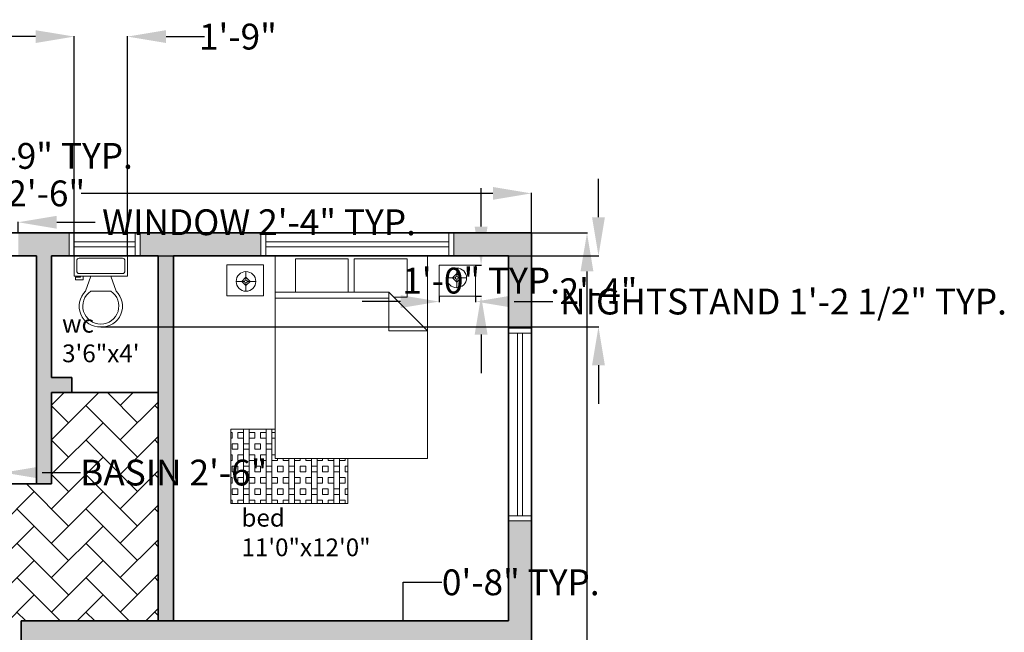
# Model space of a CAD drawing. Units: inches. Extents: x 1031 to 1706, y 87 to 654.
# Tile 4 of 4: x 1318 to 1706, y 413 to 654. Entities that reach past the tile are written whole.
import ezdxf

# ---------------------------------------------------------------- set-up
doc = ezdxf.new("R2010")
doc.units = ezdxf.units.IN
doc.header["$MEASUREMENT"] = 0
for name, color, linetype, lineweight in [('A-ANNO-DIMS', 2, 'Continuous', 18), ('A-AREA-IDEN', 7, 'Continuous', 25), ('A-FLOR-FIXT', 114, 'Continuous', 18), ('A-FLOR-PATT', 152, 'Continuous', 13), ('A-FURN', 215, 'Continuous', 18), ('A-GLAZ', 4, 'Continuous', 18), ('A-WALL', 7, 'Continuous', 35), ('A-WALL-PATT', 18, 'Continuous', 13)]:
    doc.layers.add(name, color=color, linetype=linetype, lineweight=lineweight)
doc.styles.get("Standard").update_dxf_attribs({"font": 'arial.ttf'})
doc.dimstyles.get("Standard").update_dxf_attribs({"dimtxt": 10.18, "dimasz": 15.18, "dimexe": 0.18, "dimexo": 0.0625, "dimgap": 0.09, "dimtad": 0, "dimtih": 1, "dimtoh": 1, "dimdec": 0, "dimzin": 0, "dimdsep": 46, "dimlunit": 3, "dimtxsty": 'Standard', "dimcen": 0.09, "dimadec": 0, "dimazin": 0, "dimtfac": 1, "dimtdec": 0, "dimtofl": 0, "dimtmove": 0, "dimatfit": 3, "dimfxl": 1, "dimtolj": 1, "dimtzin": 0, "dimarcsym": 0})

# ---------------------------------------------------------------- blocks, each defined once
blk = doc.blocks.new('Bed - Queen')
for p, q in [((0, -80.00003), (0, 0)), ((0, 0), (59.99999, 0)), ((59.99999, 0), (59.99999, -80.00003)), ((7.99999, -1.2), (28.79998, -1.2)), ((7.99999, -14.4), (7.99999, -1.2)), ((28.79998, -1.2), (28.79998, -14.4)), ((31.19999, -1.2), (51.99999, -1.2)), ((31.19999, -14.4), (31.19999, -1.2)), ((51.99999, -1.2), (51.99999, -16.4)), ((0, -14.4), (44.8, -14.4)), ((59.99999, -29.6), (44.8, -14.4)), ((44.8, -14.4), (44.8, -29.6)), ((44.8, -16.8), (0, -16.8)), ((51.99999, -16.4), (46.79936, -16.4)), ((44.8, -29.6), (59.99999, -29.6)), ((59.99999, -80.00003), (0, -80.00003))]:
    blk.add_line(p, q)
blk = doc.blocks.new('Lamp - Table')
for p, q in [((-1, 0), (-7, 0)), ((0, 3), (-3, 0)), ((-3, 0), (0, -3)), ((0, 7), (0, 1)), ((3, 0), (0, 3)), ((0, -3), (3, 0)), ((1, 0), (7, 0)), ((0, -1), (0, -7))]:
    blk.add_line(p, q)
for radius in [7, 1]:
    blk.add_circle((0, 0), radius)
blk = doc.blocks.new('*U11')
for p, q in [((9.5, -6), (9.5, -2)), ((-10, -8.5), (-8, -8.5)), ((-10, -9.5), (-10, -8.5)), ((-7, -9.5), (-10, -9.5)), ((-8, -8.5), (-8, -8)), ((-7, -8), (-7, -9.5)), ((-4, -8), (-6, -14)), ((4, -8), (6, -14)), ((4, -14), (-4, -14))]:
    blk.add_line(p, q)
blk.add_lwpolyline([(10.5, -8), (10.5, 0), (-10.5, 0), (-10.5, -8)], close=True)
for points in [[(-9.5, -2), (-9.5, -6)], [(8.5, -1), (-8.5, -1)], [(-8.5, -7), (8.5, -7)]]:
    blk.add_lwpolyline(points)
for centre, radius, start, end in [((-8.625, -1.875), 0.8839, 81.8699, 188.1301), ((8.625, -1.875), 0.8839, 351.8699, 98.1301), ((-8.625, -6.125), 0.8839, 171.869898, 278.1301), ((8.625, -6.125), 0.8839, 261.8699, 8.1301), ((-0.4772, -19.9188), 8.0953, 133.01722, 273.38), ((0.0374, -19.8731), 7.127, 124.50543, 269.7), ((-0.0373, -19.8731), 7.127, 270.3, 55.4946), ((0.4773, -19.9188), 8.0953, 266.62, 46.9828)]:
    blk.add_arc(centre, radius, start, end)
blk = doc.blocks.new('*D12')
at = {"layer": 'A-ANNO-DIMS', "color": 0, "lineweight": -2, "transparency": 16777216}
for p, q in [((1129.6, 570.46), (1129.6, 586.16)), ((1144.78, 585.98), (1307.03, 585.98)), ((1504.42, 585.98), (1342.17, 585.98)), ((1519.6, 570.46), (1519.6, 586.16))]:
    blk.add_line(p, q, dxfattribs=at)
at = {"layer": 'A-ANNO-DIMS', "color": 0, "transparency": 16777216}
for points in [[(1144.78, 588.51), (1144.78, 583.45), (1129.6, 585.98)], [(1504.42, 588.51), (1504.42, 583.45), (1519.6, 585.98)]]:
    blk.add_solid(points, dxfattribs=at)
at = {"layer": 'Defpoints', "color": 0, "transparency": 16777216}
for p in [(1519.6, 585.98), (1129.6, 570.4), (1519.6, 570.4)]:
    blk.add_point(p, dxfattribs=at)
at = {"layer": 'A-ANNO-DIMS', "color": 0, "transparency": 16777216, "insert": (1324.6, 585.98), "char_height": 10.18, "attachment_point": 5}
blk.add_mtext('\\A1;32\'-6"', dxfattribs=at)
blk = doc.blocks.new('*D14')
at = {"layer": 'A-ANNO-DIMS', "color": 0, "lineweight": -2, "transparency": 16777216}
for p, q in [((1519.66, 570.4), (1541.66, 570.4)), ((1541.48, 555.22), (1541.48, 383.69)), ((1541.48, 201.58), (1541.48, 373.11)), ((1519.66, 186.4), (1541.66, 186.4))]:
    blk.add_line(p, q, dxfattribs=at)
at = {"layer": 'A-ANNO-DIMS', "color": 0, "transparency": 16777216}
for points in [[(1538.95, 555.22), (1544.01, 555.22), (1541.48, 570.4)], [(1538.95, 201.58), (1544.01, 201.58), (1541.48, 186.4)]]:
    blk.add_solid(points, dxfattribs=at)
at = {"layer": 'Defpoints', "color": 0, "transparency": 16777216}
for p in [(1519.6, 570.4), (1519.6, 186.4), (1541.48, 186.4)]:
    blk.add_point(p, dxfattribs=at)
at = {"layer": 'A-ANNO-DIMS', "color": 0, "transparency": 16777216, "insert": (1541.48, 378.4), "char_height": 10.18, "attachment_point": 5}
blk.add_mtext("\\A1;32'", dxfattribs=at)
blk = doc.blocks.new('WIN-72IN')
for p, q in [((0, 0), (0, 9)), ((2, 0), (2, 9)), ((74, 0), (74, 9)), ((76, 0), (76, 9)), ((2, 5.5), (74, 5.5)), ((2, 3.5), (74, 3.5))]:
    blk.add_line(p, q)
blk = doc.blocks.new('WIN-24IN')
for p, q in [((0, 0), (0, 9)), ((2, 0), (2, 9)), ((26, 0), (26, 9)), ((28, 0), (28, 9)), ((2, 5.5), (26, 5.5)), ((2, 3.5), (26, 3.5))]:
    blk.add_line(p, q)
blk = doc.blocks.new('NIGHTSTAND-RECT')
blk.add_lwpolyline([(0, 12.21), (14.36, 12.21), (14.36, 0), (0, 0)], close=True)
blk = doc.blocks.new('*D20')
at = {"layer": 'A-ANNO-DIMS', "color": 0, "lineweight": -2, "transparency": 16777216}
for p, q in [((1274.24, 574.6), (1259.06, 574.6)), ((1289.42, 570.46), (1289.42, 574.78)), ((1317.42, 570.46), (1317.42, 574.78)), ((1332.6, 574.6), (1347.78, 574.6))]:
    blk.add_line(p, q, dxfattribs=at)
at = {"layer": 'A-ANNO-DIMS', "color": 0, "transparency": 16777216}
for points in [[(1274.24, 577.13), (1274.24, 572.07), (1289.42, 574.6)], [(1332.6, 577.13), (1332.6, 572.07), (1317.42, 574.6)]]:
    blk.add_solid(points, dxfattribs=at)
at = {"layer": 'Defpoints', "color": 0, "transparency": 16777216}
for p in [(1317.42, 574.6), (1289.42, 570.4), (1317.42, 570.4)]:
    blk.add_point(p, dxfattribs=at)
at = {"layer": 'A-ANNO-DIMS', "color": 0, "transparency": 16777216, "insert": (1412.28, 574.6), "char_height": 10.18, "attachment_point": 5}
blk.add_mtext('\\A1;WINDOW 2\'-4" TYP.', dxfattribs=at)
blk = doc.blocks.new('*D21')
at = {"layer": 'A-ANNO-DIMS', "color": 0, "lineweight": -2, "transparency": 16777216}
for p, q in [((1285.22, 585.58), (1285.22, 600.76)), ((1285.22, 600.76), (1300.4, 600.76)), ((1289.36, 570.4), (1285.04, 570.4)), ((1289.36, 561.4), (1285.04, 561.4)), ((1285.22, 546.22), (1285.22, 531.04))]:
    blk.add_line(p, q, dxfattribs=at)
at = {"layer": 'A-ANNO-DIMS', "color": 0, "transparency": 16777216}
for points in [[(1282.69, 585.58), (1287.75, 585.58), (1285.22, 570.4)], [(1282.69, 546.22), (1287.75, 546.22), (1285.22, 561.4)]]:
    blk.add_solid(points, dxfattribs=at)
at = {"layer": 'Defpoints', "color": 0, "transparency": 16777216}
for p in [(1285.22, 570.4), (1289.42, 570.4), (1289.42, 561.4)]:
    blk.add_point(p, dxfattribs=at)
at = {"layer": 'A-ANNO-DIMS', "color": 0, "transparency": 16777216, "insert": (1331.51, 600.76), "char_height": 10.18, "attachment_point": 5}
blk.add_mtext('\\A1;0\'-9" TYP.', dxfattribs=at)
blk = doc.blocks.new('*D24')
at = {"layer": 'A-ANNO-DIMS', "color": 0, "lineweight": -2, "transparency": 16777216}
for p, q in [((1468.08, 543.32), (1452.9, 543.32)), ((1483.26, 545.42), (1483.26, 543.14)), ((1497.62, 545.42), (1497.62, 543.14)), ((1512.8, 543.32), (1527.98, 543.32))]:
    blk.add_line(p, q, dxfattribs=at)
at = {"layer": 'A-ANNO-DIMS', "color": 0, "transparency": 16777216}
for points in [[(1468.08, 545.85), (1468.08, 540.79), (1483.26, 543.32)], [(1512.8, 545.85), (1512.8, 540.79), (1497.62, 543.32)]]:
    blk.add_solid(points, dxfattribs=at)
at = {"layer": 'Defpoints', "color": 0, "transparency": 16777216}
for p in [(1483.26, 545.48), (1497.62, 545.48), (1497.62, 543.32)]:
    blk.add_point(p, dxfattribs=at)
at = {"layer": 'A-ANNO-DIMS', "color": 0, "transparency": 16777216, "insert": (1618.9, 543.32), "char_height": 10.18, "attachment_point": 5}
blk.add_mtext('\\A1;NIGHTSTAND 1\'-2 1/2" TYP.', dxfattribs=at)
blk = doc.blocks.new('*D25')
at = {"layer": 'A-ANNO-DIMS', "color": 0, "lineweight": -2, "transparency": 16777216}
for p, q in [((1499.77, 572.86), (1499.77, 588.04)), ((1497.68, 557.68), (1499.95, 557.68)), ((1497.68, 545.48), (1499.95, 545.48)), ((1499.77, 530.3), (1499.77, 515.12))]:
    blk.add_line(p, q, dxfattribs=at)
at = {"layer": 'A-ANNO-DIMS', "color": 0, "transparency": 16777216}
for points in [[(1497.24, 572.86), (1502.3, 572.86), (1499.77, 557.68)], [(1497.24, 530.3), (1502.3, 530.3), (1499.77, 545.48)]]:
    blk.add_solid(points, dxfattribs=at)
at = {"layer": 'Defpoints', "color": 0, "transparency": 16777216}
for p in [(1497.62, 557.68), (1499.77, 557.68), (1497.62, 545.48)]:
    blk.add_point(p, dxfattribs=at)
at = {"layer": 'A-ANNO-DIMS', "color": 0, "transparency": 16777216, "insert": (1499.77, 551.58), "char_height": 10.18, "attachment_point": 5}
blk.add_mtext('\\A1;1\'-0" TYP.', dxfattribs=at)
blk = doc.blocks.new('*D26')
at = {"layer": 'A-ANNO-DIMS', "color": 0, "lineweight": -2, "transparency": 16777216}
for p, q in [((1455.08, 403.42), (1439.9, 403.42)), ((1470.26, 402.32), (1470.26, 403.6)), ((1478.02, 402.32), (1478.02, 403.6)), ((1493.2, 403.42), (1508.38, 403.42))]:
    blk.add_line(p, q, dxfattribs=at)
at = {"layer": 'A-ANNO-DIMS', "color": 0, "transparency": 16777216}
for points in [[(1455.08, 405.95), (1455.08, 400.89), (1470.26, 403.42)], [(1493.2, 405.95), (1493.2, 400.89), (1478.02, 403.42)]]:
    blk.add_solid(points, dxfattribs=at)
at = {"layer": 'Defpoints', "color": 0, "transparency": 16777216}
for p in [(1478.02, 403.42), (1470.26, 402.26), (1478.02, 402.26)]:
    blk.add_point(p, dxfattribs=at)
at = {"layer": 'A-ANNO-DIMS', "color": 0, "transparency": 16777216, "insert": (1560.61, 403.42), "char_height": 10.18, "attachment_point": 5}
blk.add_mtext('\\A1;LAMP 0\'-8" TYP.', dxfattribs=at)
blk = doc.blocks.new('*D27')
at = {"layer": 'A-ANNO-DIMS', "color": 0, "lineweight": -2, "transparency": 16777216}
for p, q in [((1469.1, 417.44), (1469.1, 432.62)), ((1469.1, 432.62), (1484.28, 432.62)), ((1470.2, 402.26), (1468.92, 402.26)), ((1470.2, 394.5), (1468.92, 394.5)), ((1469.1, 379.32), (1469.1, 364.14))]:
    blk.add_line(p, q, dxfattribs=at)
at = {"layer": 'A-ANNO-DIMS', "color": 0, "transparency": 16777216}
for points in [[(1466.57, 417.44), (1471.63, 417.44), (1469.1, 402.26)], [(1466.57, 379.32), (1471.63, 379.32), (1469.1, 394.5)]]:
    blk.add_solid(points, dxfattribs=at)
at = {"layer": 'Defpoints', "color": 0, "transparency": 16777216}
for p in [(1469.1, 402.26), (1470.26, 402.26), (1470.26, 394.5)]:
    blk.add_point(p, dxfattribs=at)
at = {"layer": 'A-ANNO-DIMS', "color": 0, "transparency": 16777216, "insert": (1515.39, 432.62), "char_height": 10.18, "attachment_point": 5}
blk.add_mtext('\\A1;0\'-8" TYP.', dxfattribs=at)
blk = doc.blocks.new('*D32')
at = {"layer": 'A-ANNO-DIMS', "color": 0, "lineweight": -2, "transparency": 16777216}
for p, q in [((1266.45, 475.89), (1251.27, 475.89)), ((1281.63, 471.45), (1281.63, 476.07)), ((1311.63, 471.45), (1311.63, 476.07)), ((1326.81, 475.89), (1341.99, 475.89))]:
    blk.add_line(p, q, dxfattribs=at)
at = {"layer": 'A-ANNO-DIMS', "color": 0, "transparency": 16777216}
for points in [[(1266.45, 478.42), (1266.45, 473.36), (1281.63, 475.89)], [(1326.81, 478.42), (1326.81, 473.36), (1311.63, 475.89)]]:
    blk.add_solid(points, dxfattribs=at)
at = {"layer": 'Defpoints', "color": 0, "transparency": 16777216}
for p in [(1311.63, 475.89), (1281.63, 471.39), (1311.63, 471.39)]:
    blk.add_point(p, dxfattribs=at)
at = {"layer": 'A-ANNO-DIMS', "color": 0, "transparency": 16777216, "insert": (1378.7, 475.89), "char_height": 10.18, "attachment_point": 5}
blk.add_mtext('\\A1;BASIN 2\'-6"', dxfattribs=at)
blk = doc.blocks.new('*D41')
at = {"layer": 'A-ANNO-DIMS', "color": 0, "lineweight": -2, "transparency": 16777216}
for p, q in [((1129.54, 570.4), (1054.03, 570.4)), ((1054.21, 555.22), (1054.21, 354.79)), ((1054.21, 143.78), (1054.21, 344.21)), ((1324.54, 128.6), (1054.03, 128.6))]:
    blk.add_line(p, q, dxfattribs=at)
at = {"layer": 'A-ANNO-DIMS', "color": 0, "transparency": 16777216}
for points in [[(1051.68, 555.22), (1056.74, 555.22), (1054.21, 570.4)], [(1051.68, 143.78), (1056.74, 143.78), (1054.21, 128.6)]]:
    blk.add_solid(points, dxfattribs=at)
at = {"layer": 'Defpoints', "color": 0, "transparency": 16777216}
for p in [(1054.21, 570.4), (1129.6, 570.4), (1324.6, 128.6)]:
    blk.add_point(p, dxfattribs=at)
at = {"layer": 'A-ANNO-DIMS', "color": 0, "transparency": 16777216, "insert": (1054.21, 349.5), "char_height": 10.18, "attachment_point": 5}
blk.add_mtext('\\A1;36\'-10"', dxfattribs=at)
blk = doc.blocks.new('*D44')
at = {"layer": 'A-ANNO-DIMS', "color": 0, "lineweight": -2, "transparency": 16777216}
for p, q in [((1324.29, 647.8), (1309.11, 647.8)), ((1339.47, 561.46), (1339.47, 647.98)), ((1360.47, 561.46), (1360.47, 647.98)), ((1375.65, 647.8), (1390.83, 647.8))]:
    blk.add_line(p, q, dxfattribs=at)
at = {"layer": 'A-ANNO-DIMS', "color": 0, "transparency": 16777216}
for points in [[(1324.29, 650.33), (1324.29, 645.27), (1339.47, 647.8)], [(1375.65, 650.33), (1375.65, 645.27), (1360.47, 647.8)]]:
    blk.add_solid(points, dxfattribs=at)
at = {"layer": 'Defpoints', "color": 0, "transparency": 16777216}
for p in [(1360.47, 647.8), (1339.47, 561.4), (1360.47, 561.4)]:
    blk.add_point(p, dxfattribs=at)
at = {"layer": 'A-ANNO-DIMS', "color": 0, "transparency": 16777216, "insert": (1403.97, 647.8), "char_height": 10.18, "attachment_point": 5}
blk.add_mtext('\\A1;1\'-9"', dxfattribs=at)
blk = doc.blocks.new('*D45')
at = {"layer": 'A-ANNO-DIMS', "color": 0, "lineweight": -2, "transparency": 16777216}
for p, q in [((1546.001934, 576.577381), (1546.001934, 591.757381)), ((1360.53552, 561.397381), (1546.181934, 561.397381)), ((1350.035599, 533.397413), (1546.181934, 533.397413)), ((1546.001934, 518.217413), (1546.001934, 503.037413))]:
    blk.add_line(p, q, dxfattribs=at)
at = {"layer": 'A-ANNO-DIMS', "color": 0, "transparency": 16777216}
for points in [[(1543.471934, 576.577381), (1548.531934, 576.577381), (1546.001934, 561.397381)], [(1543.471934, 518.217413), (1548.531934, 518.217413), (1546.001934, 533.397413)]]:
    blk.add_solid(points, dxfattribs=at)
at = {"layer": 'Defpoints', "color": 0, "transparency": 16777216}
for p in [(1360.47302, 561.397381), (1349.973099, 533.397413), (1546.001934, 533.397413)]:
    blk.add_point(p, dxfattribs=at)
at = {"layer": 'A-ANNO-DIMS', "color": 0, "transparency": 16777216, "insert": (1546.001934, 547.397397), "char_height": 10.18, "attachment_point": 5}
blk.add_mtext('\\A1;2\'-4"', dxfattribs=at)

msp = doc.modelspace()

# ---------------------------------------------------------------- hatches: boundary and pattern name
at = {"layer": 'A-FLOR-PATT'}
h = msp.add_hatch(dxfattribs=at)
h.set_pattern_fill('AR-HBONE', color=256, scale=2.4)
h.paths.add_polyline_path([(1372.6, 507.4), (1330.6, 507.4), (1330.6, 471.4), (1276.6, 471.4), (1276.6, 408.4), (1276.6, 336.4), (1318.6, 336.4), (1318.6, 417.4), (1372.6, 417.4)])
h = msp.add_hatch(dxfattribs=at)
h.set_pattern_fill('BOX', color=256, scale=8.9)
h.paths.add_polyline_path([(1447.25, 481.4), (1418.62, 481.4), (1418.62, 492.98), (1401.15, 492.98), (1401.15, 463.75), (1447.25, 463.75)])
at = {"layer": 'A-WALL-PATT'}
h = msp.add_hatch(color=256, dxfattribs=at)
h.dxf.hatch_style = 1
h.paths.add_polyline_path([(1324.6, 336.4), (1318.6, 336.4), (1318.6, 327.4), (1318.6, 195.4), (1256.53, 195.4), (1256.53, 186.4), (1316.43, 186.4), (1316.43, 128.6), (1324.6, 128.6), (1324.6, 142.78), (1421.89, 142.78), (1421.89, 143.49), (1324.6, 143.49), (1324.6, 157.67), (1324.6, 171.8), (1421.89, 171.8), (1421.89, 172.21), (1324.6, 172.21), (1324.6, 186.4)])
h.paths.add_polyline_path([(1378.07, 258.4), (1358.04, 258.4), (1358.04, 249.4), (1378.07, 249.4)], flags=17)
h.paths.add_polyline_path([(1519.6, 299.69), (1510.6, 299.69), (1510.6, 258.4), (1454.07, 258.4), (1454.07, 249.4), (1519.6, 249.4)])
h.paths.add_polyline_path([(1519.6, 456.87), (1510.6, 456.87), (1510.6, 417.4), (1372.6, 417.4), (1318.6, 417.4), (1318.6, 408.4), (1510.6, 408.4), (1510.6, 375.69), (1519.6, 375.69)])
h.paths.add_polyline_path([(1276.6, 372.4), (1270.65, 372.4), (1270.65, 336.4), (1138.6, 336.4), (1092.08, 336.4), (1092.08, 346.4), (1080.61, 346.4), (1080.61, 327.4), (1129.6, 327.4), (1129.6, 290.93), (1138.6, 290.93), (1138.6, 291.84), (1138.6, 327.4), (1244.94, 327.4), (1276.6, 327.4)])
h.paths.add_polyline_path([(1276.6, 417.4), (1138.6, 417.4), (1138.6, 438.03), (1129.6, 438.03), (1129.6, 417.4), (1080.61, 417.4), (1080.61, 398.4), (1092.08, 398.4), (1092.08, 408.4), (1138.6, 408.4), (1276.6, 408.4)])
h.paths.add_polyline_path([(1180.53, 195.4), (1138.6, 195.4), (1138.6, 214.93), (1129.6, 214.93), (1129.6, 186.4), (1180.53, 186.4)])
h.paths.add_polyline_path([(1519.6, 570.4), (1489.02, 570.4), (1489.02, 561.4), (1510.6, 561.4), (1510.6, 532.87), (1519.6, 532.87)])
h.paths.add_polyline_path([(1413.02, 570.4), (1365.47, 570.4), (1365.47, 561.4), (1372.6, 561.4), (1372.6, 507.4), (1372.6, 417.4), (1378.6, 417.4), (1378.6, 561.4), (1413.02, 561.4)])
h.paths.add_polyline_path([(1289.42, 570.4), (1242.6, 570.4), (1242.6, 561.4), (1270.6, 561.4), (1270.6, 471.4), (1291.02, 471.4), (1291.02, 477.4), (1276.6, 477.4), (1276.6, 561.4), (1289.42, 561.4)])
h.paths.add_polyline_path([(1337.47, 570.4), (1317.42, 570.4), (1317.42, 561.4), (1324.6, 561.4), (1324.6, 471.4), (1330.6, 471.4), (1330.6, 507.4), (1338.54, 507.4), (1338.54, 513.4), (1330.6, 513.4), (1330.6, 561.4), (1337.47, 561.4)])
h.paths.add_polyline_path([(1138.6, 561.4), (1166.6, 561.4), (1166.6, 570.4), (1129.6, 570.4), (1129.6, 514.03), (1138.6, 514.03)])

# ---------------------------------------------------------------- linework, layer by layer
at = {"layer": 'A-FURN'}
for p, q in [((1418.62, 492.98), (1401.15, 492.98)), ((1401.15, 492.98), (1401.15, 463.75)), ((1447.25, 463.75), (1447.25, 481.4)), ((1401.15, 463.75), (1447.25, 463.75))]:
    msp.add_line(p, q, dxfattribs=at)
at = {"layer": 'A-WALL'}
for p, q in [((1129.6, 570.4), (1519.6, 570.4)), ((1519.6, 570.4), (1519.6, 186.4)), ((1276.6, 561.4), (1324.6, 561.4)), ((1324.6, 471.4), (1324.6, 561.4)), ((1330.6, 561.4), (1372.6, 561.4)), ((1330.6, 513.4), (1330.6, 561.4)), ((1372.6, 507.4), (1372.6, 561.4)), ((1378.6, 417.4), (1378.6, 561.4)), ((1378.6, 561.4), (1510.6, 561.4)), ((1510.6, 561.4), (1510.6, 417.4)), ((1330.6, 513.4), (1338.54, 513.4)), ((1338.54, 513.4), (1338.54, 507.4)), ((1330.6, 507.4), (1372.6, 507.4)), ((1330.6, 471.4), (1330.6, 507.4)), ((1372.6, 417.4), (1372.6, 507.4)), ((1270.6, 471.4), (1330.6, 471.4)), ((1318.6, 417.4), (1372.6, 417.4)), ((1318.6, 327.4), (1318.6, 417.4)), ((1372.6, 417.4), (1510.6, 417.4))]:
    msp.add_line(p, q, dxfattribs=at)

# ---------------------------------------------------------------- block references
at = {"layer": 'A-FLOR-FIXT'}
msp.add_blockref('*U11', (1349.97, 561.4), dxfattribs=at)
at = {"layer": 'A-FURN'}
for name, p in [('Bed - Queen', (1418.62, 561.4)), ('NIGHTSTAND-RECT', (1399.67, 545.63)), ('NIGHTSTAND-RECT', (1483.26, 545.48))]:
    msp.add_blockref(name, p, dxfattribs=at)
at = {"layer": 'A-FURN', "xscale": 0.5540798285396209, "yscale": 0.5540798285396209, "zscale": 0.5540798285396209}
for p in [(1407.15, 551.27), (1490.17, 552.67)]:
    msp.add_blockref('Lamp - Table', p, dxfattribs=at)
at = {"layer": 'A-GLAZ'}
for name, p, rotation in [('WIN-24IN', (1365.47, 570.4), 180), ('WIN-72IN', (1489.02, 570.4), 180), ('WIN-72IN', (1519.6, 456.87), 90.0000000000009)]:
    msp.add_blockref(name, p, dxfattribs=dict(at, rotation=rotation))

# ---------------------------------------------------------------- texts
at = {"layer": 'A-AREA-IDEN', "char_height": 7, "attachment_point": 1}
for s, insert in [('wc\\P3\'6"x4\'', (1334.71, 538.07)), ('bed\\P11\'0"x12\'0"', (1405.35, 461.58))]:
    msp.add_mtext_dynamic_manual_height_columns(s, width=113.8004, gutter_width=1, heights=[0], dxfattribs=dict(at, insert=insert))

# ---------------------------------------------------------------- dimensions: what is measured, and where the dimension line sits
at = {"layer": 'A-ANNO-DIMS'}
for base, p1, p2, override, picture, middle in [((1360.47, 647.8), (1339.47, 561.4), (1360.47, 561.4), {"dimdec": 1, "dimlfac": 1, "dimrnd": 0, "dimzin": 1, "dimdsep": 46, "dimlunit": 4, "dimfrac": 2}, '*D44', (1403.97, 647.8)), ((1519.6, 585.98), (1129.6, 570.4), (1519.6, 570.4), {"dimclrd": 0, "dimclre": 0, "dimclrt": 0}, '*D12', (1324.6, 585.98))]:
    dim = msp.add_linear_dim(base=base, p1=p1, p2=p2, dimstyle='Standard', override=override, dxfattribs=at)
    dim.commit()
    dim.dimension.update_dxf_attribs({"geometry": picture, "text_midpoint": middle})
for base, p1, p2, picture, middle in [((1285.22, 570.4), (1289.42, 561.4), (1289.42, 570.4), '*D21', (1331.51, 600.76)), ((1499.77, 557.68), (1497.62, 545.48), (1497.62, 557.68), '*D25', (1499.77, 551.58)), ((1469.1, 402.26), (1470.26, 394.5), (1470.26, 402.26), '*D27', (1515.39, 432.62))]:
    dim = msp.add_linear_dim(base=base, p1=p1, p2=p2, angle=90, text='<> TYP.', dimstyle='Standard', override={"dimdec": 1, "dimlfac": 1, "dimrnd": 0, "dimzin": 1, "dimdsep": 46, "dimlunit": 4, "dimfrac": 2}, dxfattribs=at)
    dim.commit()
    dim.dimension.update_dxf_attribs({"geometry": picture, "text_midpoint": middle})
for base, p1, p2, text, picture, middle in [((1317.42, 574.6), (1289.42, 570.4), (1317.42, 570.4), 'WINDOW <> TYP.', '*D20', (1412.28, 574.6)), ((1497.62, 543.32), (1483.26, 545.48), (1497.62, 545.48), 'NIGHTSTAND <> TYP.', '*D24', (1618.9, 543.32)), ((1311.63, 475.89), (1281.63, 471.39), (1311.63, 471.39), 'BASIN <>', '*D32', (1378.7, 475.89)), ((1478.02, 403.42), (1470.26, 402.26), (1478.02, 402.26), 'LAMP <> TYP.', '*D26', (1560.61, 403.42))]:
    dim = msp.add_linear_dim(base=base, p1=p1, p2=p2, text=text, dimstyle='Standard', override={"dimdec": 1, "dimlfac": 1, "dimrnd": 0, "dimzin": 1, "dimdsep": 46, "dimlunit": 4, "dimfrac": 2}, dxfattribs=at)
    dim.commit()
    dim.dimension.update_dxf_attribs({"geometry": picture, "text_midpoint": middle})
for base, p1, p2, override, picture, middle in [((1546, 533.4), (1360.47, 561.4), (1349.97, 533.4), {"dimdec": 1, "dimlfac": 1, "dimrnd": 0, "dimzin": 1, "dimdsep": 46, "dimlunit": 4, "dimfrac": 2}, '*D45', (1546, 547.4)), ((1054.21, 570.4), (1324.6, 128.6), (1129.6, 570.4), {"dimdec": 1, "dimlfac": 1, "dimrnd": 0, "dimzin": 1, "dimdsep": 46, "dimlunit": 4, "dimfrac": 2}, '*D41', (1054.21, 349.5)), ((1541.48, 186.4), (1519.6, 570.4), (1519.6, 186.4), {"dimclrd": 0, "dimclre": 0, "dimclrt": 0}, '*D14', (1541.48, 378.4))]:
    dim = msp.add_linear_dim(base=base, p1=p1, p2=p2, angle=90, dimstyle='Standard', override=override, dxfattribs=at)
    dim.commit()
    dim.dimension.update_dxf_attribs({"geometry": picture, "text_midpoint": middle})

doc.saveas('drawing.dxf')
